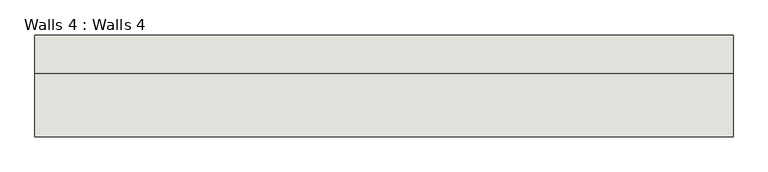
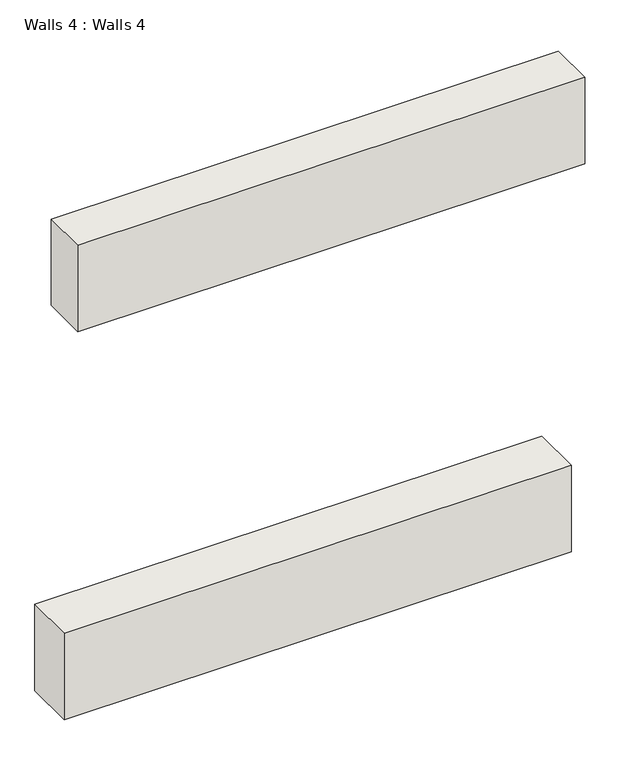
"""IFC4 building model written with IfcOpenShell, lengths in millimetres: wall geometry, Walls 4 : Walls 4."""

from ifc_helpers import new_model, si_unit, frame, origin, place, context, project, spatial, polyline, outline, extrude, source, transform, mapped, element, save


def walls_4_walls_4_ee6bbb79(model_context):
    return source(origin(), model_context, "Body", "SweptSolid", [
        extrude(outline(polyline([(-1482.6998814, 69.5610824), (-5851.4998814, 69.5610824), (-5851.4998814, 463.2610824), (-1482.6998814, 463.2610824), (-1482.6998814, 69.5610824)])), frame((0.0, 0.0, 7315.2), z_axis=(0.0, 0.0, 1.0), x_axis=(1.0, 0.0, 0.0)), (0.0, 0.0, 1.0), 786.7096072),
        extrude(outline(polyline([(-1482.6998814, 272.7610824), (-5851.4998814, 272.7610824), (-5851.4998814, 707.1064999), (-1482.6998814, 707.1064999), (-1482.6998814, 272.7610824)])), frame((0.0, 0.0, 3657.6), z_axis=(0.0, 0.0, 1.0), x_axis=(1.0, 0.0, 0.0)), (0.0, 0.0, 1.0), 786.7096072),
    ])


if __name__ == "__main__":
    model = new_model("IFC4")
    model_context = context("Model", 3, world=origin())
    ifc_project = project(units=[si_unit("LENGTHUNIT", "METRE", prefix="MILLI")], contexts=[model_context])
    site = spatial("IfcSite", under=ifc_project)
    building = spatial("IfcBuilding", under=site)
    placement = place(None, origin())
    walls_4_walls_4_shape = walls_4_walls_4_ee6bbb79(model_context)
    element("IfcWall", 1, ObjectType="Walls 4 : Walls 4", at=placement, inside=building, context=model_context, shape_type="MappedRepresentation", body=[
        mapped(walls_4_walls_4_shape, transform((0.0, 0.0, 0.0), x_axis=(1.0, 0.0, 0.0), y_axis=(0.0, 1.0, 0.0), z_axis=(0.0, 0.0, 1.0))),
    ])
    save(model, "model.ifc")

# Revit data of these elements
# Element 1 (IfcWall, "Walls 4 : Walls 4")
#   Materials on its faces: "Default Wall"
# Materials
#   "Default Wall": colour RGB 128 128 128, transparency 0
